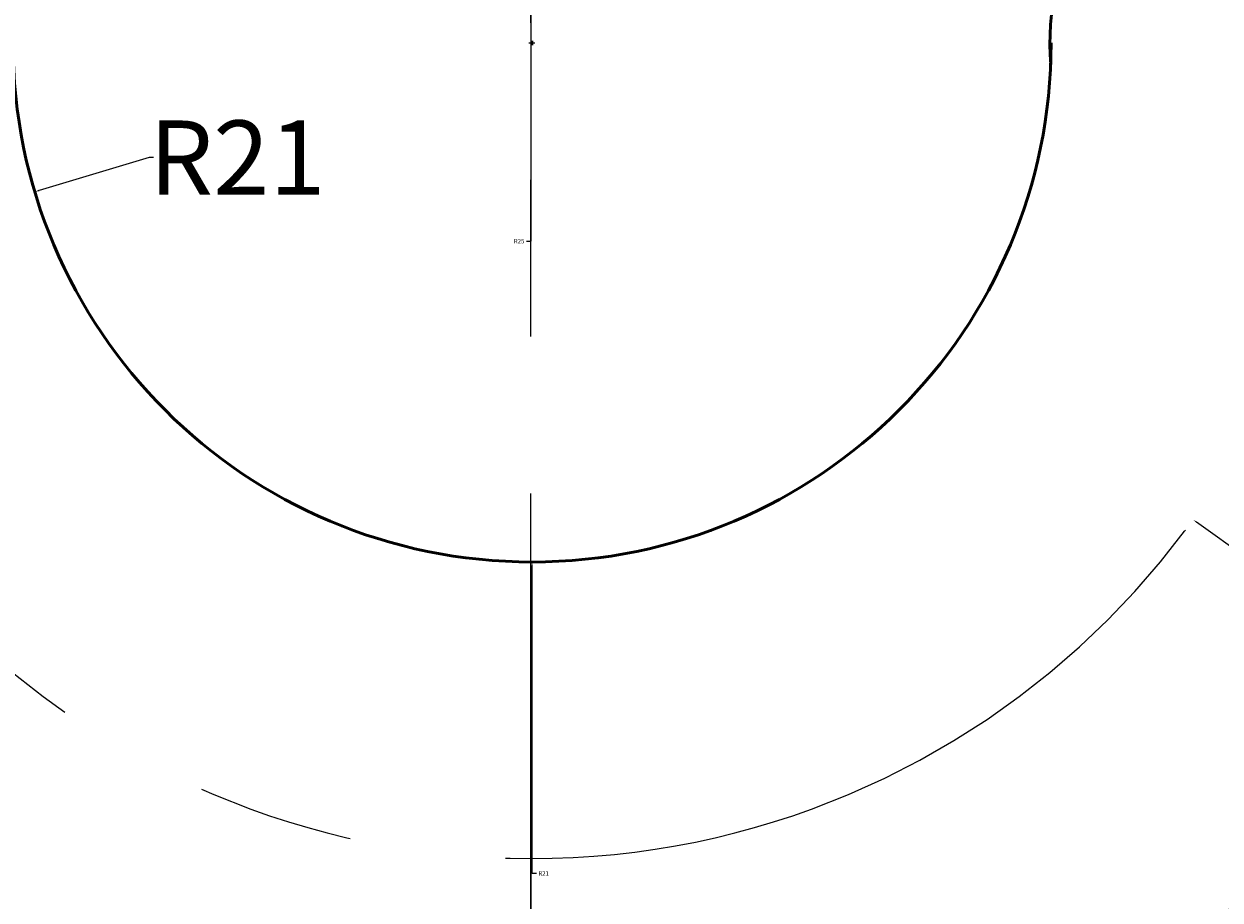
# Model space of a CAD drawing. Units: millimetres. Extents: x -50 to 109, y -46 to 152.
# Tile 12 of 18: x 13 to 61, y 32 to 67. Entities that reach past the tile are written whole.
import ezdxf

# ---------------------------------------------------------------- set-up
doc = ezdxf.new("R2010")
doc.units = ezdxf.units.MM
doc.header["$MEASUREMENT"] = 0
doc.linetypes.add('CENTER', pattern=[50.8, 31.75, -6.35, 6.35, -6.35])
for name, color, linetype, lineweight in [('M-CNTR', 1, 'CENTER', 18), ('M-DIMS', 2, 'Continuous', 25), ('M-OUTL', 7, 'Continuous', 50)]:
    doc.layers.add(name, color=color, linetype=linetype, lineweight=lineweight)
doc.styles.get("Standard").update_dxf_attribs({"font": 'arial.ttf'})
doc.dimstyles.get("Standard").update_dxf_attribs({"dimtxt": 0.18, "dimasz": 0.18, "dimexe": 0.18, "dimexo": 0.0625, "dimgap": 0.09, "dimtad": 0, "dimtih": 1, "dimtoh": 1, "dimdec": 4, "dimzin": 0, "dimdsep": 46, "dimtxsty": 'Standard', "dimcen": 0.09, "dimadec": 0, "dimazin": 0, "dimtfac": 1, "dimtdec": 4, "dimtofl": 0, "dimtmove": 0, "dimatfit": 3, "dimfxl": 1, "dimtolj": 1, "dimtzin": 0, "dimarcsym": 0})

# ---------------------------------------------------------------- blocks, each defined once
blk = doc.blocks.new('*U3')
at = {"layer": 'M-CNTR', "color": 0, "transparency": 16777216}
blk.add_line((0, -85.984), (0, -2.6), dxfattribs=at)
blk = doc.blocks.new('*D17')
at = {"layer": 'Defpoints', "color": 0, "transparency": 16777216}
for p in [(33.17, 66.25), (13.052, 60.229)]:
    blk.add_point(p, dxfattribs=at)
at = {"layer": 'M-DIMS', "color": 0, "lineweight": -2, "transparency": 16777216}
for p, q in [((17.676, 61.613), (13.224, 60.28)), ((17.856, 61.613), (17.676, 61.613))]:
    blk.add_line(p, q, dxfattribs=at)
at = {"layer": 'M-DIMS', "color": 0, "transparency": 16777216}
blk.add_solid([(13.215, 60.309), (13.233, 60.252), (13.052, 60.229)], dxfattribs=at)
at = {"layer": 'M-DIMS', "color": 0, "transparency": 16777216, "insert": (21.241, 61.613), "char_height": 0.18, "attachment_point": 5}
blk.add_mtext('\\A1;{\\H16.66667x;R21}', dxfattribs=at)
blk = doc.blocks.new('*D18')
at = {"layer": 'Defpoints', "color": 0, "transparency": 16777216}
for p in [(33.131, 66.25), (59.909, 46.965)]:
    blk.add_point(p, dxfattribs=at)
at = {"layer": 'M-DIMS', "color": 0, "lineweight": -2, "transparency": 16777216}
for p, q in [((33.131, 66.16), (33.131, 66.34)), ((33.041, 66.25), (33.221, 66.25)), ((80.717, 31.98), (60.055, 46.86)), ((80.897, 31.98), (80.717, 31.98))]:
    blk.add_line(p, q, dxfattribs=at)
at = {"layer": 'M-DIMS', "color": 0, "transparency": 16777216}
blk.add_solid([(60.073, 46.884), (60.038, 46.835), (59.909, 46.965)], dxfattribs=at)
at = {"layer": 'M-DIMS', "color": 0, "transparency": 16777216, "insert": (84.571, 31.98), "char_height": 0.18, "attachment_point": 5}
blk.add_mtext('\\A1;{\\H16.66667x;R33}', dxfattribs=at)
blk = doc.blocks.new('*D28')
at = {"layer": 'Defpoints', "color": 0, "transparency": 16777216}
for p in [(33.197, 66.25), (78.068, 62.85)]:
    blk.add_point(p, dxfattribs=at)
at = {"layer": 'M-DIMS', "color": 0, "lineweight": -2, "transparency": 16777216}
for p, q in [((33.197, 66.16), (33.197, 66.34)), ((33.107, 66.25), (33.287, 66.25)), ((102.361, 61.009), (78.248, 62.836))]:
    blk.add_line(p, q, dxfattribs=at)
at = {"layer": 'M-DIMS', "color": 0, "transparency": 16777216}
blk.add_solid([(78.25, 62.866), (78.246, 62.806), (78.068, 62.85)], dxfattribs=at)
at = {"layer": 'M-DIMS', "color": 0, "transparency": 16777216, "insert": (106.046, 61.009), "char_height": 0.18, "attachment_point": 5}
blk.add_mtext('\\A1;{\\H16.66667x;R45}', dxfattribs=at)
blk = doc.blocks.new('*D35')
at = {"layer": 'Defpoints', "color": 0, "transparency": 16777216}
for p in [(33.17, 66.25), (33.17, 45.25)]:
    blk.add_point(p, dxfattribs=at)
at = {"layer": 'M-DIMS', "color": 0, "lineweight": -2, "transparency": 16777216}
for p, q in [((33.17, 66.16), (33.17, 66.34)), ((33.08, 66.25), (33.26, 66.25)), ((33.17, 32.65), (33.17, 45.07)), ((33.35, 32.65), (33.17, 32.65))]:
    blk.add_line(p, q, dxfattribs=at)
at = {"layer": 'M-DIMS', "color": 0, "transparency": 16777216}
blk.add_solid([(33.2, 45.07), (33.14, 45.07), (33.17, 45.25)], dxfattribs=at)
at = {"layer": 'M-DIMS', "color": 0, "transparency": 16777216, "insert": (33.638, 32.65), "char_height": 0.18, "attachment_point": 5}
blk.add_mtext('\\A1;R21', dxfattribs=at)
blk = doc.blocks.new('*D37')
at = {"layer": 'Defpoints', "color": 0, "transparency": 16777216}
for p in [(33.132, 98.231), (33.131, 73.231)]:
    blk.add_point(p, dxfattribs=at)
at = {"layer": 'M-DIMS', "color": 0, "lineweight": -2, "transparency": 16777216}
for p, q in [((33.132, 98.141), (33.132, 98.321)), ((33.042, 98.231), (33.222, 98.231)), ((33.13, 58.231), (33.131, 73.051)), ((32.95, 58.231), (33.13, 58.231))]:
    blk.add_line(p, q, dxfattribs=at)
at = {"layer": 'M-DIMS', "color": 0, "transparency": 16777216}
blk.add_solid([(33.101, 73.051), (33.161, 73.051), (33.131, 73.231)], dxfattribs=at)
at = {"layer": 'M-DIMS', "color": 0, "transparency": 16777216, "insert": (32.645, 58.231), "char_height": 0.18, "attachment_point": 5}
blk.add_mtext('\\A1;R25', dxfattribs=at)
blk = doc.blocks.new('*D38')
at = {"layer": 'Defpoints', "color": 0, "transparency": 16777216}
for p in [(33.131, 66.25), (33.131, 33.25)]:
    blk.add_point(p, dxfattribs=at)
at = {"layer": 'M-DIMS', "color": 0, "lineweight": -2, "transparency": 16777216}
for p, q in [((33.131, 66.16), (33.131, 66.34)), ((33.041, 66.25), (33.221, 66.25)), ((33.131, 13.45), (33.131, 33.07)), ((33.311, 13.45), (33.131, 13.45))]:
    blk.add_line(p, q, dxfattribs=at)
at = {"layer": 'M-DIMS', "color": 0, "transparency": 16777216}
blk.add_solid([(33.161, 33.07), (33.101, 33.07), (33.131, 33.25)], dxfattribs=at)
at = {"layer": 'M-DIMS', "color": 0, "transparency": 16777216, "insert": (33.616, 13.45), "char_height": 0.18, "attachment_point": 5}
blk.add_mtext('\\A1;R33', dxfattribs=at)
blk = doc.blocks.new('*D39')
at = {"layer": 'Defpoints', "color": 0, "transparency": 16777216}
for p in [(33.197, 66.25), (33.197, 21.25)]:
    blk.add_point(p, dxfattribs=at)
at = {"layer": 'M-DIMS', "color": 0, "lineweight": -2, "transparency": 16777216}
for p, q in [((33.197, 66.16), (33.197, 66.34)), ((33.107, 66.25), (33.287, 66.25)), ((33.197, -5.75), (33.197, 21.07)), ((33.017, -5.75), (33.197, -5.75))]:
    blk.add_line(p, q, dxfattribs=at)
at = {"layer": 'M-DIMS', "color": 0, "transparency": 16777216}
blk.add_solid([(33.167, 21.07), (33.227, 21.07), (33.197, 21.25)], dxfattribs=at)
at = {"layer": 'M-DIMS', "color": 0, "transparency": 16777216, "insert": (32.711, -5.75), "char_height": 0.18, "attachment_point": 5}
blk.add_mtext('\\A1;R45', dxfattribs=at)

msp = doc.modelspace()

# ---------------------------------------------------------------- linework, layer by layer
at = {"layer": 'M-CNTR'}
msp.add_arc((33.1307, 66.24997), 33, 180.014282, 359.985718, dxfattribs=at)
at = {"layer": 'M-OUTL'}
msp.add_line((54.12333, 66.24174), (54.16988, 66.24174), dxfattribs=at)
for centre, radius, start, end in [((0.13105, 66.18507), 21, 44.15899, 179.845381), ((66.1299, 66.18218), 21, 0.162515, 135.835986), ((66.12325, 66.19749), 12, 0.211276, 183.937929), ((33.197, 66.24997), 45, 180.010473, 359.989527), ((33.16988, 66.24975), 21, 180, 0)]:
    msp.add_arc(centre, radius, start, end, dxfattribs=at)

# ---------------------------------------------------------------- block references
at = {"layer": 'M-CNTR'}
msp.add_blockref('*U3', (33.11888, 102.25066), dxfattribs=at)

# ---------------------------------------------------------------- dimensions: what is measured, and where the dimension line sits
at = {"layer": 'M-DIMS'}
for center, mpoint, picture, middle in [((33.13188, 98.23105), (33.131, 73.23105), '*D37', (32.64474, 58.23105)), ((33.197, 66.24997), (33.197, 21.24997), '*D39', (32.71127, -5.75003)), ((33.1307, 66.24997), (33.131, 33.24997), '*D38', (33.61623, 13.44997)), ((33.16988, 66.24975), (33.17, 45.24975), '*D35', (33.63775, 32.64975))]:
    dim = msp.add_radius_dim(center=center, mpoint=mpoint, dimstyle='Standard', override={"dimdec": 0, "dimlfac": 1, "dimrnd": 0, "dimzin": 0, "dimdsep": 46, "dimlunit": 2}, dxfattribs=at)
    dim.commit()
    dim.dimension.update_dxf_attribs({"geometry": picture, "text_midpoint": middle, "dimtype": 164})
for center, mpoint, text, picture, middle in [((33.1307, 66.24997), (59.90911, 46.96483), '{\\H16.66667x;R33}', '*D18', (84.57118, 31.97955)), ((33.197, 66.24997), (78.06836, 62.8499), '{\\H16.66667x;R45}', '*D28', (102.36058, 61.0092)), ((33.16988, 66.24975), (13.05155, 60.22873), '{\\H16.66667x;R21}', '*D17', (21.24115, 61.61288))]:
    dim = msp.add_radius_dim(center=center, mpoint=mpoint, text=text, dimstyle='Standard', override={"dimclrd": 0, "dimclre": 0, "dimclrt": 0}, dxfattribs=at)
    dim.commit()
    dim.dimension.update_dxf_attribs({"geometry": picture, "text_midpoint": middle, "dimtype": 164})

doc.saveas('drawing.dxf')
